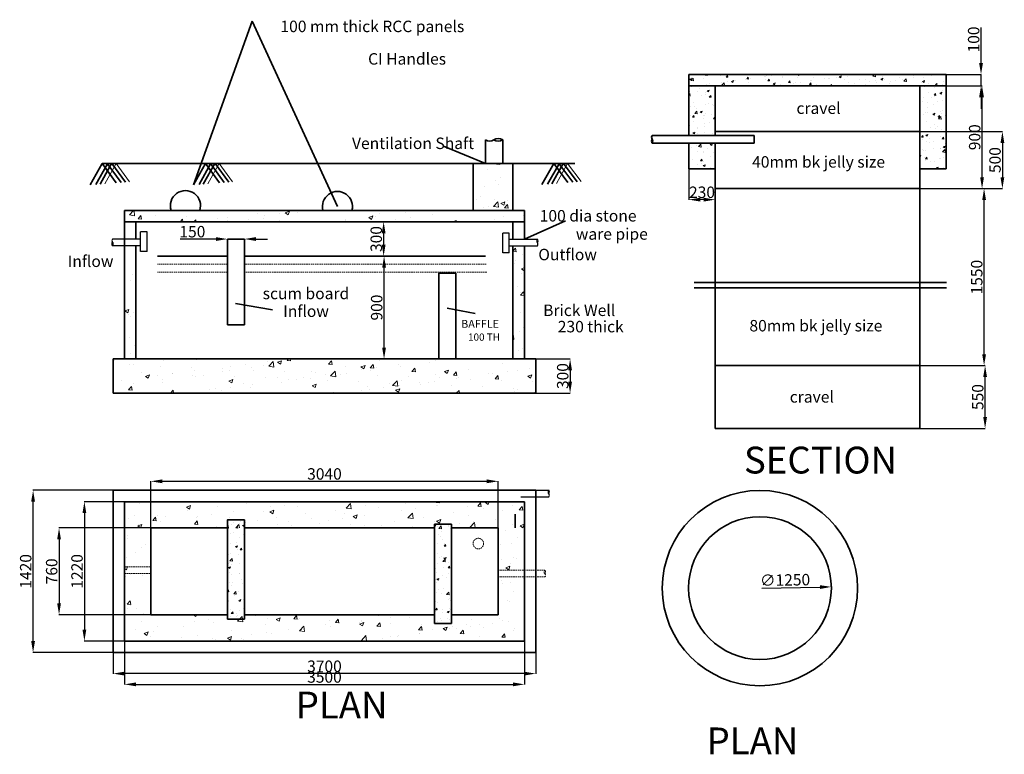
# Model space of a CAD drawing. Units: metres. Extents: x 669 to 9289, y -327 to 6106.
import ezdxf

# ---------------------------------------------------------------- set-up
doc = ezdxf.new("R2010")
doc.units = ezdxf.units.M
doc.linetypes.add('DASHED', pattern=[19.05, 12.7, -6.35])
for name, color, linetype, lineweight in [('A-ANNO-DIMS', 2, 'Continuous', 18), ('A-ANNO-TEXT', 7, 'Continuous', 25), ('A-DETL', 7, 'Continuous', 35), ('A-DETL-HIDN', 4, 'DASHED', 18), ('A-DETL-PATT', 8, 'Continuous', 13), ('C-TOPO', 8, 'Continuous', 18), ('P-SANR-PIPE', 3, 'Continuous', 25)]:
    doc.layers.add(name, color=color, linetype=linetype, lineweight=lineweight)
doc.styles.get("Standard").update_dxf_attribs({"font": 'arial.ttf'})
doc.dimstyles.new('ISO-25', dxfattribs={"dimtxt": 100, "dimasz": 100, "dimexe": 1.25, "dimexo": 0.625, "dimtad": 1, "dimdec": 0, "dimtxsty": 'Standard', "dimcen": 2.5, "dimadec": 0, "dimazin": 0, "dimtfac": 1, "dimtdec": 0, "dimtmove": 0, "dimatfit": 3, "dimfxl": 1, "dimarcsym": 0})

# ---------------------------------------------------------------- blocks, each defined once
blk = doc.blocks.new('*D1')
at = {"layer": 'A-ANNO-DIMS', "color": 0, "lineweight": -2, "transparency": 16777216}
for p, q in [((1487.3, 564.8), (1487.3, 378.7)), ((5187.3, 564.8), (5187.3, 378.7)), ((5087.3, 380), (1587.3, 380))]:
    blk.add_line(p, q, dxfattribs=at)
at = {"layer": 'A-ANNO-DIMS', "color": 0, "transparency": 16777216}
for points in [[(1587.3, 396.6), (1587.3, 363.3), (1487.3, 380)], [(5087.3, 396.6), (5087.3, 363.3), (5187.3, 380)]]:
    blk.add_solid(points, dxfattribs=at)
at = {"layer": 'Defpoints', "color": 0, "transparency": 16777216}
for p in [(1487.3, 565.4), (5187.3, 565.4), (1487.3, 380)]:
    blk.add_point(p, dxfattribs=at)
at = {"layer": 'A-ANNO-DIMS', "color": 0, "transparency": 16777216, "insert": (3337.3, 431.7), "char_height": 100, "attachment_point": 5}
blk.add_mtext('3700', dxfattribs=at)
blk = doc.blocks.new('*D2')
at = {"layer": 'A-ANNO-DIMS', "color": 0, "lineweight": -2, "transparency": 16777216}
for p, q in [((1817.3, 896), (1817.3, 2065.2)), ((1917.3, 2063.9), (4757.3, 2063.9)), ((4857.3, 896), (4857.3, 2065.2))]:
    blk.add_line(p, q, dxfattribs=at)
at = {"layer": 'A-ANNO-DIMS', "color": 0, "transparency": 16777216}
for points in [[(1917.3, 2080.6), (1917.3, 2047.2), (1817.3, 2063.9)], [(4757.3, 2080.6), (4757.3, 2047.2), (4857.3, 2063.9)]]:
    blk.add_solid(points, dxfattribs=at)
at = {"layer": 'Defpoints', "color": 0, "transparency": 16777216}
for p in [(4857.3, 2063.9), (1817.3, 895.4), (4857.3, 895.4)]:
    blk.add_point(p, dxfattribs=at)
at = {"layer": 'A-ANNO-DIMS', "color": 0, "transparency": 16777216, "insert": (3337.3, 2115.6), "char_height": 100, "attachment_point": 5}
blk.add_mtext('3040', dxfattribs=at)
blk = doc.blocks.new('*D3')
at = {"layer": 'A-ANNO-DIMS', "color": 0, "lineweight": -2, "transparency": 16777216}
for p, q in [((1587.3, 664.8), (1587.3, 284.6)), ((5087.3, 664.8), (5087.3, 284.6)), ((1687.3, 285.8), (4987.3, 285.8))]:
    blk.add_line(p, q, dxfattribs=at)
at = {"layer": 'A-ANNO-DIMS', "color": 0, "transparency": 16777216}
for points in [[(1687.3, 302.5), (1687.3, 269.1), (1587.3, 285.8)], [(4987.3, 302.5), (4987.3, 269.1), (5087.3, 285.8)]]:
    blk.add_solid(points, dxfattribs=at)
at = {"layer": 'Defpoints', "color": 0, "transparency": 16777216}
for p in [(1587.3, 665.4), (5087.3, 665.4), (5087.3, 285.8)]:
    blk.add_point(p, dxfattribs=at)
at = {"layer": 'A-ANNO-DIMS', "color": 0, "transparency": 16777216, "insert": (3337.3, 337.5), "char_height": 100, "attachment_point": 5}
blk.add_mtext('3500', dxfattribs=at)
blk = doc.blocks.new('*D4')
at = {"layer": 'A-ANNO-DIMS', "color": 0, "lineweight": -2, "transparency": 16777216}
for p, q in [((1816.7, 1655.4), (1012.7, 1655.4)), ((1013.9, 1555.4), (1013.9, 995.4)), ((1816.7, 895.4), (1012.7, 895.4))]:
    blk.add_line(p, q, dxfattribs=at)
at = {"layer": 'A-ANNO-DIMS', "color": 0, "transparency": 16777216}
for points in [[(997.3, 1555.4), (1030.6, 1555.4), (1013.9, 1655.4)], [(997.3, 995.4), (1030.6, 995.4), (1013.9, 895.4)]]:
    blk.add_solid(points, dxfattribs=at)
at = {"layer": 'Defpoints', "color": 0, "transparency": 16777216}
for p in [(1817.3, 1655.4), (1013.9, 895.4), (1817.3, 895.4)]:
    blk.add_point(p, dxfattribs=at)
at = {"layer": 'A-ANNO-DIMS', "color": 0, "transparency": 16777216, "insert": (962.2, 1275.4), "char_height": 100, "attachment_point": 5, "rotation": 90}
blk.add_mtext('760', dxfattribs=at)
blk = doc.blocks.new('*D5')
at = {"layer": 'A-ANNO-DIMS', "color": 0, "lineweight": -2, "transparency": 16777216}
for p, q in [((1586.7, 1885.4), (1234.5, 1885.4)), ((1235.7, 1785.4), (1235.7, 765.4)), ((1586.7, 665.4), (1234.5, 665.4))]:
    blk.add_line(p, q, dxfattribs=at)
at = {"layer": 'A-ANNO-DIMS', "color": 0, "transparency": 16777216}
for points in [[(1219.1, 1785.4), (1252.4, 1785.4), (1235.7, 1885.4)], [(1219.1, 765.4), (1252.4, 765.4), (1235.7, 665.4)]]:
    blk.add_solid(points, dxfattribs=at)
at = {"layer": 'Defpoints', "color": 0, "transparency": 16777216}
for p in [(1587.3, 1885.4), (1235.7, 665.4), (1587.3, 665.4)]:
    blk.add_point(p, dxfattribs=at)
at = {"layer": 'A-ANNO-DIMS', "color": 0, "transparency": 16777216, "insert": (1184.1, 1275.4), "char_height": 100, "attachment_point": 5, "rotation": 90}
blk.add_mtext('1220', dxfattribs=at)
blk = doc.blocks.new('*D6')
at = {"layer": 'A-ANNO-DIMS', "color": 0, "lineweight": -2, "transparency": 16777216}
for p, q in [((1486.7, 1985.4), (785.3, 1985.4)), ((786.6, 665.4), (786.6, 1885.4)), ((1486.7, 565.4), (785.3, 565.4))]:
    blk.add_line(p, q, dxfattribs=at)
at = {"layer": 'A-ANNO-DIMS', "color": 0, "transparency": 16777216}
for points in [[(769.9, 1885.4), (803.2, 1885.4), (786.6, 1985.4)], [(769.9, 665.4), (803.2, 665.4), (786.6, 565.4)]]:
    blk.add_solid(points, dxfattribs=at)
at = {"layer": 'Defpoints', "color": 0, "transparency": 16777216}
for p in [(786.6, 1985.4), (1487.3, 1985.4), (1487.3, 565.4)]:
    blk.add_point(p, dxfattribs=at)
at = {"layer": 'A-ANNO-DIMS', "color": 0, "transparency": 16777216, "insert": (734.9, 1275.4), "char_height": 100, "attachment_point": 5, "rotation": 90}
blk.add_mtext('1420', dxfattribs=at)
blk = doc.blocks.new('*D7')
at = {"layer": 'A-ANNO-DIMS', "color": 0, "lineweight": -2, "transparency": 16777216}
blk.add_line((7166.3, 1129), (7674.6, 1137.7), dxfattribs=at)
at = {"layer": 'A-ANNO-DIMS', "color": 0, "transparency": 16777216}
blk.add_solid([(7674.3, 1154.3), (7674.9, 1121), (7774.6, 1139.4)], dxfattribs=at)
at = {"layer": 'Defpoints', "color": 0, "transparency": 16777216}
for p in [(7774.6, 1139.4), (6524.8, 1118.1)]:
    blk.add_point(p, dxfattribs=at)
at = {"layer": 'A-ANNO-DIMS', "color": 0, "transparency": 16777216, "insert": (7369.6, 1187), "char_height": 100, "attachment_point": 5, "rotation": 0.97303}
blk.add_mtext('∅1250', dxfattribs=at)
blk = doc.blocks.new('*D8')
at = {"layer": 'A-ANNO-DIMS', "color": 0, "lineweight": -2, "transparency": 16777216}
for p, q in [((8549.8, 3076.8), (9121.9, 3076.8)), ((9120.6, 2626.8), (9120.6, 2976.8)), ((8549.8, 2526.8), (9121.9, 2526.8))]:
    blk.add_line(p, q, dxfattribs=at)
at = {"layer": 'A-ANNO-DIMS', "color": 0, "transparency": 16777216}
for points in [[(9104, 2976.8), (9137.3, 2976.8), (9120.6, 3076.8)], [(9104, 2626.8), (9137.3, 2626.8), (9120.6, 2526.8)]]:
    blk.add_solid(points, dxfattribs=at)
at = {"layer": 'Defpoints', "color": 0, "transparency": 16777216}
for p in [(8549.2, 3076.8), (9120.6, 3076.8), (8549.2, 2526.8)]:
    blk.add_point(p, dxfattribs=at)
at = {"layer": 'A-ANNO-DIMS', "color": 0, "transparency": 16777216, "insert": (9069, 2801.8), "char_height": 100, "attachment_point": 5, "rotation": 90}
blk.add_mtext('550', dxfattribs=at)
blk = doc.blocks.new('*D9')
at = {"layer": 'A-ANNO-DIMS', "color": 0, "lineweight": -2, "transparency": 16777216}
for p, q in [((8549.8, 4626.8), (9113, 4626.8)), ((9111.7, 3176.8), (9111.7, 4526.8)), ((8549.8, 3076.8), (9113, 3076.8))]:
    blk.add_line(p, q, dxfattribs=at)
at = {"layer": 'A-ANNO-DIMS', "color": 0, "transparency": 16777216}
for points in [[(9095.1, 4526.8), (9128.4, 4526.8), (9111.7, 4626.8)], [(9095.1, 3176.8), (9128.4, 3176.8), (9111.7, 3076.8)]]:
    blk.add_solid(points, dxfattribs=at)
at = {"layer": 'Defpoints', "color": 0, "transparency": 16777216}
for p in [(8549.2, 4626.8), (9111.7, 4626.8), (8549.2, 3076.8)]:
    blk.add_point(p, dxfattribs=at)
at = {"layer": 'A-ANNO-DIMS', "color": 0, "transparency": 16777216, "insert": (9060.1, 3851.8), "char_height": 100, "attachment_point": 5, "rotation": 90}
blk.add_mtext('1550', dxfattribs=at)
blk = doc.blocks.new('*D10')
at = {"layer": 'A-ANNO-DIMS', "color": 0, "lineweight": -2, "transparency": 16777216}
for p, q in [((8549.8, 5526.8), (9095.2, 5526.8)), ((9093.9, 4726.8), (9093.9, 5426.8)), ((8549.8, 4626.8), (9095.2, 4626.8))]:
    blk.add_line(p, q, dxfattribs=at)
at = {"layer": 'A-ANNO-DIMS', "color": 0, "transparency": 16777216}
for points in [[(9077.3, 5426.8), (9110.6, 5426.8), (9093.9, 5526.8)], [(9077.3, 4726.8), (9110.6, 4726.8), (9093.9, 4626.8)]]:
    blk.add_solid(points, dxfattribs=at)
at = {"layer": 'Defpoints', "color": 0, "transparency": 16777216}
for p in [(8549.2, 5526.8), (9093.9, 5526.8), (8549.2, 4626.8)]:
    blk.add_point(p, dxfattribs=at)
at = {"layer": 'A-ANNO-DIMS', "color": 0, "transparency": 16777216, "insert": (9042.2, 5076.8), "char_height": 100, "attachment_point": 5, "rotation": 90}
blk.add_mtext('900', dxfattribs=at)
blk = doc.blocks.new('*D11')
at = {"layer": 'A-ANNO-DIMS', "color": 0, "lineweight": -2, "transparency": 16777216}
for p, q in [((8549.8, 5126.8), (9273.3, 5126.8)), ((9272.1, 5026.8), (9272.1, 4726.8)), ((8549.8, 4626.8), (9273.3, 4626.8))]:
    blk.add_line(p, q, dxfattribs=at)
at = {"layer": 'A-ANNO-DIMS', "color": 0, "transparency": 16777216}
for points in [[(9255.4, 5026.8), (9288.7, 5026.8), (9272.1, 5126.8)], [(9255.4, 4726.8), (9288.7, 4726.8), (9272.1, 4626.8)]]:
    blk.add_solid(points, dxfattribs=at)
at = {"layer": 'Defpoints', "color": 0, "transparency": 16777216}
for p in [(8549.2, 5126.8), (8549.2, 4626.8), (9272.1, 4626.8)]:
    blk.add_point(p, dxfattribs=at)
at = {"layer": 'A-ANNO-DIMS', "color": 0, "transparency": 16777216, "insert": (9220.4, 4876.8), "char_height": 100, "attachment_point": 5, "rotation": 90}
blk.add_mtext('500', dxfattribs=at)
blk = doc.blocks.new('*D12')
at = {"layer": 'A-ANNO-DIMS', "color": 0, "lineweight": -2, "transparency": 16777216}
for p, q in [((9085, 5726.8), (9085, 6039.2)), ((8779.8, 5626.8), (9086.3, 5626.8)), ((9085, 5526.8), (9085, 5626.8)), ((8779.8, 5526.8), (9086.3, 5526.8)), ((9085, 5426.8), (9085, 5326.8))]:
    blk.add_line(p, q, dxfattribs=at)
at = {"layer": 'A-ANNO-DIMS', "color": 0, "transparency": 16777216}
for points in [[(9068.3, 5726.8), (9101.7, 5726.8), (9085, 5626.8)], [(9068.3, 5426.8), (9101.7, 5426.8), (9085, 5526.8)]]:
    blk.add_solid(points, dxfattribs=at)
at = {"layer": 'Defpoints', "color": 0, "transparency": 16777216}
for p in [(8779.2, 5626.8), (9085, 5626.8), (8779.2, 5526.8)]:
    blk.add_point(p, dxfattribs=at)
at = {"layer": 'A-ANNO-DIMS', "color": 0, "transparency": 16777216, "insert": (9033.3, 5933), "char_height": 100, "attachment_point": 5, "rotation": 90}
blk.add_mtext('100', dxfattribs=at)
blk = doc.blocks.new('*D13')
at = {"layer": 'A-ANNO-DIMS', "color": 0, "lineweight": -2, "transparency": 16777216}
for p, q in [((6527.4, 4800.2), (6527.4, 4529.2)), ((6757.4, 4800.2), (6757.4, 4529.2)), ((6657.4, 4530.5), (6627.4, 4530.5))]:
    blk.add_line(p, q, dxfattribs=at)
at = {"layer": 'A-ANNO-DIMS', "color": 0, "transparency": 16777216}
for points in [[(6627.4, 4547.1), (6627.4, 4513.8), (6527.4, 4530.5)], [(6657.4, 4547.1), (6657.4, 4513.8), (6757.4, 4530.5)]]:
    blk.add_solid(points, dxfattribs=at)
at = {"layer": 'Defpoints', "color": 0, "transparency": 16777216}
for p in [(6527.4, 4800.8), (6757.4, 4800.8), (6527.4, 4530.5)]:
    blk.add_point(p, dxfattribs=at)
at = {"layer": 'A-ANNO-DIMS', "color": 0, "transparency": 16777216, "insert": (6642.4, 4582.2), "char_height": 100, "attachment_point": 5}
blk.add_mtext('230', dxfattribs=at)
blk = doc.blocks.new('*D14')
at = {"layer": 'A-ANNO-DIMS', "color": 0, "lineweight": -2, "transparency": 16777216}
for p, q in [((4747.7, 4035.4), (3857.8, 4035.4)), ((3859, 3235.4), (3859, 3935.4)), ((5186.7, 3135.4), (3857.8, 3135.4))]:
    blk.add_line(p, q, dxfattribs=at)
at = {"layer": 'A-ANNO-DIMS', "color": 0, "transparency": 16777216}
for points in [[(3842.3, 3935.4), (3875.7, 3935.4), (3859, 4035.4)], [(3842.3, 3235.4), (3875.7, 3235.4), (3859, 3135.4)]]:
    blk.add_solid(points, dxfattribs=at)
at = {"layer": 'Defpoints', "color": 0, "transparency": 16777216}
for p in [(3859, 4035.4), (4748.3, 4035.4), (5187.3, 3135.4)]:
    blk.add_point(p, dxfattribs=at)
at = {"layer": 'A-ANNO-DIMS', "color": 0, "transparency": 16777216, "insert": (3807.3, 3585.4), "char_height": 100, "attachment_point": 5, "rotation": 90}
blk.add_mtext('900', dxfattribs=at)
blk = doc.blocks.new('*D15')
at = {"layer": 'A-ANNO-DIMS', "color": 0, "lineweight": -2, "transparency": 16777216}
for p, q in [((5086.7, 4335.4), (3854, 4335.4)), ((3855.3, 4235.4), (3855.3, 4135.4)), ((3848, 4035.4), (3856.5, 4035.4))]:
    blk.add_line(p, q, dxfattribs=at)
at = {"layer": 'A-ANNO-DIMS', "color": 0, "transparency": 16777216}
for points in [[(3838.6, 4235.4), (3871.9, 4235.4), (3855.3, 4335.4)], [(3838.6, 4135.4), (3871.9, 4135.4), (3855.3, 4035.4)]]:
    blk.add_solid(points, dxfattribs=at)
at = {"layer": 'Defpoints', "color": 0, "transparency": 16777216}
for p in [(5087.3, 4335.4), (3847.3, 4035.4), (3855.3, 4035.4)]:
    blk.add_point(p, dxfattribs=at)
at = {"layer": 'A-ANNO-DIMS', "color": 0, "transparency": 16777216, "insert": (3803.6, 4185.4), "char_height": 100, "attachment_point": 5, "rotation": 90}
blk.add_mtext('300', dxfattribs=at)
blk = doc.blocks.new('*D16')
at = {"layer": 'A-ANNO-DIMS', "color": 0, "lineweight": -2, "transparency": 16777216}
for p, q in [((2387.3, 4185.4), (2074.9, 4185.4)), ((2487.3, 4186), (2487.3, 4186.6)), ((2637.3, 4185.4), (2487.3, 4185.4)), ((2637.3, 4186), (2637.3, 4186.6)), ((2737.3, 4185.4), (2837.3, 4185.4))]:
    blk.add_line(p, q, dxfattribs=at)
at = {"layer": 'A-ANNO-DIMS', "color": 0, "transparency": 16777216}
for points in [[(2387.3, 4202), (2387.3, 4168.7), (2487.3, 4185.4)], [(2737.3, 4202), (2737.3, 4168.7), (2637.3, 4185.4)]]:
    blk.add_solid(points, dxfattribs=at)
at = {"layer": 'Defpoints', "color": 0, "transparency": 16777216}
for p in [(2487.3, 4185.4), (2487.3, 4185.4), (2637.3, 4185.4)]:
    blk.add_point(p, dxfattribs=at)
at = {"layer": 'A-ANNO-DIMS', "color": 0, "transparency": 16777216, "insert": (2181.1, 4237), "char_height": 100, "attachment_point": 5}
blk.add_mtext('150', dxfattribs=at)
blk = doc.blocks.new('*D17')
at = {"layer": 'A-ANNO-DIMS', "color": 0, "lineweight": -2, "transparency": 16777216}
for p, q in [((5187.9, 3135.4), (5488.8, 3135.4)), ((5487.6, 3035.4), (5487.6, 2935.4)), ((5187.9, 2835.4), (5488.8, 2835.4))]:
    blk.add_line(p, q, dxfattribs=at)
at = {"layer": 'A-ANNO-DIMS', "color": 0, "transparency": 16777216}
for points in [[(5470.9, 3035.4), (5504.2, 3035.4), (5487.6, 3135.4)], [(5470.9, 2935.4), (5504.2, 2935.4), (5487.6, 2835.4)]]:
    blk.add_solid(points, dxfattribs=at)
at = {"layer": 'Defpoints', "color": 0, "transparency": 16777216}
for p in [(5187.3, 3135.4), (5187.3, 2835.4), (5487.6, 2835.4)]:
    blk.add_point(p, dxfattribs=at)
at = {"layer": 'A-ANNO-DIMS', "color": 0, "transparency": 16777216, "insert": (5435.9, 2985.4), "char_height": 100, "attachment_point": 5, "rotation": 90}
blk.add_mtext('300', dxfattribs=at)
blk = doc.blocks.new('PIPE-END')
for p, q in [((252.1, 58.6), (6, 58.6)), ((252.1, 0), (6, 0))]:
    blk.add_line(p, q)
for centre, radius, start, end in [((24.5, 16.1), 24.5, 138.99016, 221.00984), ((19.8, 45.4), 19.1, 136.11307, 223.88693), ((-11.5, 16.1), 23.7, 317.36785, 42.63215)]:
    blk.add_arc(centre, radius, start, end)
blk = doc.blocks.new('BAFFLE-WALL-PLAN')
for p, q in [((150, 869.9), (0, 869.9)), ((0, 869.9), (0, 750)), ((150, 750), (150, 869.9)), ((0, 750), (0, 0)), ((150, 750), (150, 0)), ((150, 0), (0, 0))]:
    blk.add_line(p, q)
blk = doc.blocks.new('PIPE-COLLAR')
for p, q in [((0, 0), (0, 173)), ((57.7, 173), (0, 173)), ((57.7, 0), (57.7, 173)), ((57.7, 0), (0, 0))]:
    blk.add_line(p, q)
blk = doc.blocks.new('GROUND-SYMB')
for p, q in [((98.9, 175.4), (0, 0)), ((215.8, 16.4), (98.9, 175.4))]:
    blk.add_line(p, q)

msp = doc.modelspace()

# ---------------------------------------------------------------- hatches: boundary and pattern name
at = {"layer": 'A-DETL-PATT'}
h = msp.add_hatch(dxfattribs=at)
h.set_pattern_fill('AR-CONC', color=256)
h.paths.add_polyline_path([(8779.2, 5626.8), (8549.2, 5626.8), (6757.4, 5626.8), (6527.4, 5626.8), (6527.4, 5526.8), (8779.2, 5526.8)])
h.paths.add_polyline_path([(6757.4, 5526.8), (6527.4, 5526.8), (6527.4, 5092.8), (6757.4, 5092.8)])
h.paths.add_polyline_path([(6757.4, 5025.9), (6527.4, 5025.9), (6527.4, 4800.8), (6757.4, 4800.8)])
h.paths.add_polyline_path([(8779.2, 5526.8), (8549.2, 5526.8), (8549.2, 4800.8), (8779.2, 4800.8)])
h = msp.add_hatch(dxfattribs=at)
h.set_pattern_fill('AR-CONC', color=256, scale=2)
h.paths.add_polyline_path([(4987.3, 4845.5), (4639.3, 4845.5), (4639.3, 4435.4), (4987.3, 4435.4)])
h = msp.add_hatch(dxfattribs=at)
h.set_pattern_fill('AR-CONC', color=256, scale=2)
h.paths.add_polyline_path([(5087.3, 4435.4), (1587.3, 4435.4), (1587.3, 4335.4), (5087.3, 4335.4)])
h.paths.add_polyline_path([(1687.3, 4126.7), (1587.3, 4126.7), (1587.3, 3135.4), (1687.3, 3135.4)])
h.paths.add_polyline_path([(5187.3, 3135.4), (1487.3, 3135.4), (1487.3, 2835.4), (5187.3, 2835.4)])
h.paths.add_polyline_path([(5087.3, 4127), (4987.3, 4127), (4987.3, 3135.4), (5087.3, 3135.4)])
h.paths.add_polyline_path([(5087.3, 1885.4), (1587.3, 1885.4), (1587.3, 665.4), (5087.3, 665.4)])
h.paths.add_polyline_path([(4857.3, 1655.4), (4857.3, 895.4), (1817.3, 895.4), (1817.3, 1655.4)], flags=16)
h = msp.add_hatch(dxfattribs=at)
h.set_pattern_fill('AR-CONC', color=256)
h.paths.add_polyline_path([(2638.3, 1607.3), (2638.3, 1727.1), (2488.3, 1727.1), (2488.3, 1607.3), (2488.3, 857.3), (2638.3, 857.3)])
h.paths.add_polyline_path([(4450.5, 1569.6), (4450.5, 1689.5), (4300.5, 1689.5), (4300.5, 1569.6), (4300.5, 819.6), (4450.5, 819.6)])

# ---------------------------------------------------------------- linework, layer by layer
at = {"layer": 'A-DETL'}
for p, q in [((2190.6, 4660.5), (2704, 6094.5)), ((2704, 6094.5), (3451.2, 4470.2)), ((6527.4, 5626.8), (6757.4, 5626.8)), ((6527.4, 5626.8), (6527.4, 5626.8)), ((6527.4, 5092.8), (6527.4, 5626.8)), ((8549.2, 5626.8), (6757.4, 5626.8)), ((8549.2, 5626.8), (8779.2, 5626.8)), ((8779.2, 5626.8), (8779.2, 4800.8)), ((8779.2, 5526.8), (6527.4, 5526.8)), ((6757.4, 5092.8), (6757.4, 5526.8)), ((8549.2, 4626.8), (8549.2, 5526.8)), ((7100.3, 5092.8), (6205.7, 5092.8)), ((8549.2, 5126.8), (6757.4, 5126.8)), ((7100.3, 5092.8), (7100.3, 5025.9)), ((4748, 5053.6), (4748, 4845.5)), ((4898, 5053.6), (4898, 4845.5)), ((7100.3, 5025.9), (6205.7, 5025.9)), ((6527.4, 4800.8), (6527.4, 5025.9)), ((6757.4, 2526.8), (6757.4, 5025.9)), ((4378.7, 4998.6), (4748, 4845.5)), ((1391.8, 4845.5), (1287.5, 4660.5)), ((1391.8, 4845.5), (1287.5, 4660.5)), ((1437.5, 4843.5), (1336.4, 4664.2)), ((1474.3, 4845.5), (1373.7, 4667)), ((4639.3, 4845.5), (1391.8, 4845.5)), ((1515.1, 4677.8), (1391.8, 4845.5)), ((1515.1, 4677.8), (1391.8, 4845.5)), ((1515.1, 4677.8), (1391.8, 4845.5)), ((1515.1, 4677.8), (1391.8, 4845.5)), ((1515.1, 4677.8), (1391.8, 4845.5)), ((1557, 4680.9), (1436, 4845.5)), ((1595.7, 4683.9), (1476.9, 4845.5)), ((2294.9, 4845.5), (2190.6, 4660.5)), ((2294.9, 4845.5), (2190.6, 4660.5)), ((2340.6, 4843.5), (2239.5, 4664.2)), ((2377.4, 4845.5), (2276.8, 4667)), ((2418.2, 4677.8), (2294.9, 4845.5)), ((2418.2, 4677.8), (2294.9, 4845.5)), ((2418.2, 4677.8), (2294.9, 4845.5)), ((2418.2, 4677.8), (2294.9, 4845.5)), ((2418.2, 4677.8), (2294.9, 4845.5)), ((2460.1, 4680.9), (2339.1, 4845.5)), ((2498.8, 4683.9), (2380, 4845.5)), ((4987.3, 4845.5), (4639.3, 4845.5)), ((4639.3, 4845.5), (4639.3, 4435.4)), ((4987.3, 4435.4), (4987.3, 4845.5)), ((4987.3, 4845.5), (5242.1, 4845.5)), ((5345.2, 4847.1), (5241, 4662.1)), ((5345.2, 4847.1), (5241, 4662.1)), ((5242.1, 4845.5), (5242.1, 4845.5)), ((5242.1, 4845.5), (5529.9, 4845.5)), ((5390.9, 4845.1), (5289.8, 4665.8)), ((5427.8, 4847.1), (5327.2, 4668.6)), ((5468.5, 4679.3), (5345.2, 4847.1)), ((5468.5, 4679.3), (5345.2, 4847.1)), ((5468.5, 4679.3), (5345.2, 4847.1)), ((5468.5, 4679.3), (5345.2, 4847.1)), ((5468.5, 4679.3), (5345.2, 4847.1)), ((5510.4, 4682.5), (5389.5, 4847.1)), ((5549.2, 4685.5), (5430.4, 4847.1)), ((6527.4, 4800.8), (6757.4, 4800.8)), ((8779.2, 4800.8), (8549.2, 4800.8)), ((8549.2, 4626.8), (6757.4, 4626.8)), ((8549.2, 3076.8), (8549.2, 4626.8)), ((1587.3, 4435.4), (1587.3, 3135.4)), ((5087.3, 4435.4), (1587.3, 4435.4)), ((1587.3, 4435.4), (1587.3, 4185.4)), ((5087.3, 4185.6), (5087.3, 4435.4)), ((5087.3, 4335.4), (1587.3, 4335.4)), ((1687.3, 4335.4), (1687.3, 4185.4)), ((4987.3, 4185.6), (4987.3, 4335.4)), ((5446, 4344.6), (5087.3, 4185.6)), ((2637.3, 4185.4), (2487.3, 4185.4)), ((2487.3, 4185.4), (2487.3, 3435.4)), ((2637.3, 4185.4), (2637.3, 3435.4)), ((1687.3, 4126.7), (1687.3, 3135.4)), ((4987.3, 3135.4), (4987.3, 4127)), ((5087.3, 3135.4), (5087.3, 4127)), ((2487.3, 4035.4), (1874.7, 4035.4)), ((4748.3, 4035.4), (2637.3, 4035.4)), ((4337.3, 3135.4), (4337.3, 3885.4)), ((4487.3, 3885.4), (4337.3, 3885.4)), ((4487.3, 3135.4), (4487.3, 3885.4)), ((6572.6, 3805.2), (8781.4, 3805.2)), ((6572.6, 3757.3), (8781.4, 3757.3)), ((2881.9, 3564.5), (2559.6, 3621.2)), ((4655.9, 3534.8), (4411.9, 3580.1)), ((2637.3, 3435.4), (2487.3, 3435.4)), ((5187.3, 3135.4), (1487.3, 3135.4)), ((1487.3, 3135.4), (1487.3, 2835.4)), ((5187.3, 2835.4), (5187.3, 3135.4)), ((8549.2, 3076.8), (6757.4, 3076.8)), ((8549.2, 2526.8), (8549.2, 3076.8)), ((1487.3, 2835.4), (5187.3, 2835.4)), ((6757.4, 2526.8), (8549.2, 2526.8)), ((8549.2, 2526.8), (6757.4, 2526.8)), ((5187.3, 1985.4), (1487.3, 1985.4)), ((1487.3, 1985.4), (1487.3, 565.4)), ((5187.3, 565.4), (5187.3, 1985.4)), ((5087.3, 1885.4), (1587.3, 1885.4)), ((1587.3, 1885.4), (1587.3, 665.4)), ((5087.3, 665.4), (5087.3, 1885.4)), ((5007.3, 1655.4), (5007.3, 1775.3)), ((5007.3, 1655.4), (5007.3, 1775.3)), ((1817.3, 1655.4), (1817.3, 895.4)), ((2488.3, 1655.4), (1817.3, 1655.4)), ((1817.3, 1645.4), (1817.3, 895.4)), ((4300.5, 1655.4), (2638.3, 1655.4)), ((4857.3, 1655.4), (4450.5, 1655.4)), ((4857.3, 895.4), (4857.3, 1655.4)), ((4857.3, 1655.4), (4857.3, 905.4)), ((1817.3, 895.4), (2488.3, 895.4)), ((1967.3, 895.4), (1817.3, 895.4)), ((2638.3, 895.4), (4300.5, 895.4)), ((4450.5, 895.4), (4857.3, 895.4)), ((1587.3, 665.4), (5087.3, 665.4)), ((1487.3, 565.4), (5187.3, 565.4))]:
    msp.add_line(p, q, dxfattribs=at)
for radius in [855, 625]:
    msp.add_circle((7149.7, 1128.8), radius, dxfattribs=at)
for centre, radius, start, end in [((6229, 5076.9), 28.2, 145.69593, 214.30407), ((4783.6, 5110), 66.7, 237.72992, 302.27008), ((4858.6, 4998.8), 67.5, 54.30956, 125.69044), ((4858.6, 5110.2), 68.9, 235.16288, 304.83712), ((6236.2, 5043.5), 35.2, 150, 210), ((6175.3, 5043.5), 35.2, 330, 30), ((2120.4, 4477.7), 131.7, 341.25384, 198.74616), ((3451.2, 4470.2), 131.7, 344.67012, 195.32988), ((1796.7, 1298), 24.5, 32.61479, 41.00984)]:
    msp.add_arc(centre, radius, start, end, dxfattribs=at)
at = {"layer": 'A-DETL-HIDN'}
for p, q in [((2487.3, 3965.4), (1874.7, 3965.4)), ((4753.2, 3965.4), (2637.3, 3965.4)), ((2487.3, 3895.4), (1874.7, 3895.4)), ((4758, 3895.4), (2637.3, 3895.4)), ((1587.3, 1314), (1817.3, 1314)), ((1587.3, 1255.4), (1817.3, 1255.4)), ((4857.3, 1284.9), (5266.8, 1284.9)), ((4857.3, 1226.3), (5266.8, 1226.3))]:
    msp.add_line(p, q, dxfattribs=at)
msp.add_circle((4684.5, 1518.6), 46.1, dxfattribs=at)
for centre, radius, start, end in [((5284.3, 1268.8), 23.7, 137.36785, 222.63215), ((5248.3, 1268.8), 24.5, 318.99016, 41.00984), ((5253.1, 1239.5), 19.1, 316.11307, 43.88693)]:
    msp.add_arc(centre, radius, start, end, dxfattribs=at)

# ---------------------------------------------------------------- block references
at = {"layer": 'A-DETL'}
for p in [(2488.3, 857.3), (4300.5, 819.6)]:
    msp.add_blockref('BAFFLE-WALL-PLAN', p, dxfattribs=at)
at = {"layer": 'C-TOPO'}
for p in [(1413.9, 4670.1), (2317, 4670.1), (5367.3, 4671.7)]:
    msp.add_blockref('GROUND-SYMB', p, dxfattribs=at)
at = {"layer": 'P-SANR-PIPE'}
for name, p in [('PIPE-COLLAR', (1727.7, 4075.2)), ('PIPE-COLLAR', (4897.4, 4064.3)), ('PIPE-END', (1475.7, 4126.7))]:
    msp.add_blockref(name, p, dxfattribs=at)
at = {"layer": 'P-SANR-PIPE', "rotation": 180}
for p in [(5207.3, 4185.6), (5307.3, 1985.4)]:
    msp.add_blockref('PIPE-END', p, dxfattribs=at)

# ---------------------------------------------------------------- texts
at = {"layer": 'A-ANNO-TEXT'}
for s, height, p in [('100 mm thick RCC panels', 100.444, (2951.7, 5997.2)), ('CI Handles', 100.44, (3719.2, 5712.8)), ('cravel ', 100.44, (7469.2, 5281.1)), ('cravel ', 100.44, (7469.2, 5281.1)), ('Ventilation Shaft', 100.444, (3578.2, 4973.6)), ('40mm bk jelly size', 100.444, (7080.8, 4810.8)), ('100 dia stone ', 100.444, (5221.5, 4339)), ('ware pipe', 100.44, (5537.9, 4179.4)), ('Inflow ', 100.44, (1089.7, 3940.7)), ('Outflow', 100.44, (5209.3, 3999.5)), ('scum board ', 100.444, (2796.4, 3658.5)), ('Brick Well', 100.44, (5251.7, 3511.3)), ('Inflow ', 100.44, (2976, 3503.2)), ('BAFFLE', 69.39, (4533.8, 3408.1)), ('230 thick ', 100.44, (5379.7, 3368.4)), ('80mm bk jelly size ', 100.444, (7057.3, 3376.3)), ('100 TH', 63.5, (4594.3, 3294.9)), ('cravel ', 100.44, (7410.4, 2753.2)), ('SECTION', 234.93, (7009.7, 2132.2)), ('PLAN', 234.93, (3085.9, -12.8)), ('PLAN', 234.93, (6682.4, -326.8))]:
    msp.add_text(s, height=height, dxfattribs=at).set_placement(p)

# ---------------------------------------------------------------- dimensions: what is measured, and where the dimension line sits
at = {"layer": 'A-ANNO-DIMS'}
for base, p1, p2, picture, middle in [((9085, 5626.8), (8779.2, 5526.8), (8779.2, 5626.8), '*D12', (9033.3, 5933)), ((9093.9, 5526.8), (8549.2, 4626.8), (8549.2, 5526.8), '*D10', (9042.2, 5076.8)), ((9272.1, 4626.8), (8549.2, 5126.8), (8549.2, 4626.8), '*D11', (9220.4, 4876.8)), ((9111.7, 4626.8), (8549.2, 3076.8), (8549.2, 4626.8), '*D9', (9060.1, 3851.8)), ((3855.3, 4035.4), (5087.3, 4335.4), (3847.3, 4035.4), '*D15', (3803.6, 4185.4)), ((3859, 4035.4), (5187.3, 3135.4), (4748.3, 4035.4), '*D14', (3807.3, 3585.4)), ((5487.6, 2835.4), (5187.3, 3135.4), (5187.3, 2835.4), '*D17', (5435.9, 2985.4)), ((9120.6, 3076.8), (8549.2, 2526.8), (8549.2, 3076.8), '*D8', (9069, 2801.8)), ((786.6, 1985.4), (1487.3, 565.4), (1487.3, 1985.4), '*D6', (734.9, 1275.4)), ((1235.7, 665.4), (1587.3, 1885.4), (1587.3, 665.4), '*D5', (1184.1, 1275.4)), ((1013.9, 895.4), (1817.3, 1655.4), (1817.3, 895.4), '*D4', (962.2, 1275.4))]:
    dim = msp.add_linear_dim(base=base, p1=p1, p2=p2, angle=90, dimstyle='ISO-25', override={"dimclrd": 0, "dimclre": 0, "dimclrt": 0}, dxfattribs=at)
    dim.commit()
    dim.dimension.update_dxf_attribs({"geometry": picture, "text_midpoint": middle})
for base, p1, p2, picture, middle in [((6527.4, 4530.5), (6757.4, 4800.8), (6527.4, 4800.8), '*D13', (6642.4, 4582.2)), ((2487.3, 4185.4), (2637.3, 4185.4), (2487.3, 4185.4), '*D16', (2181.1, 4237)), ((4857.3, 2063.9), (1817.3, 895.4), (4857.3, 895.4), '*D2', (3337.3, 2115.6)), ((5087.3, 285.8), (1587.3, 665.4), (5087.3, 665.4), '*D3', (3337.3, 337.5)), ((1487.3, 380), (5187.3, 565.4), (1487.3, 565.4), '*D1', (3337.3, 431.7))]:
    dim = msp.add_linear_dim(base=base, p1=p1, p2=p2, dimstyle='ISO-25', override={"dimclrd": 0, "dimclre": 0, "dimclrt": 0}, dxfattribs=at)
    dim.commit()
    dim.dimension.update_dxf_attribs({"geometry": picture, "text_midpoint": middle})
dim = msp.add_diameter_dim_2p(p1=(6524.8, 1118.1), p2=(7774.6, 1139.4), dimstyle='ISO-25', override={"dimclrd": 0, "dimclre": 0, "dimclrt": 0}, dxfattribs=at)
dim.commit()
dim.dimension.update_dxf_attribs({"geometry": '*D7', "text_midpoint": (7370.5, 1132.5), "dimtype": 163})

doc.saveas('drawing.dxf')
